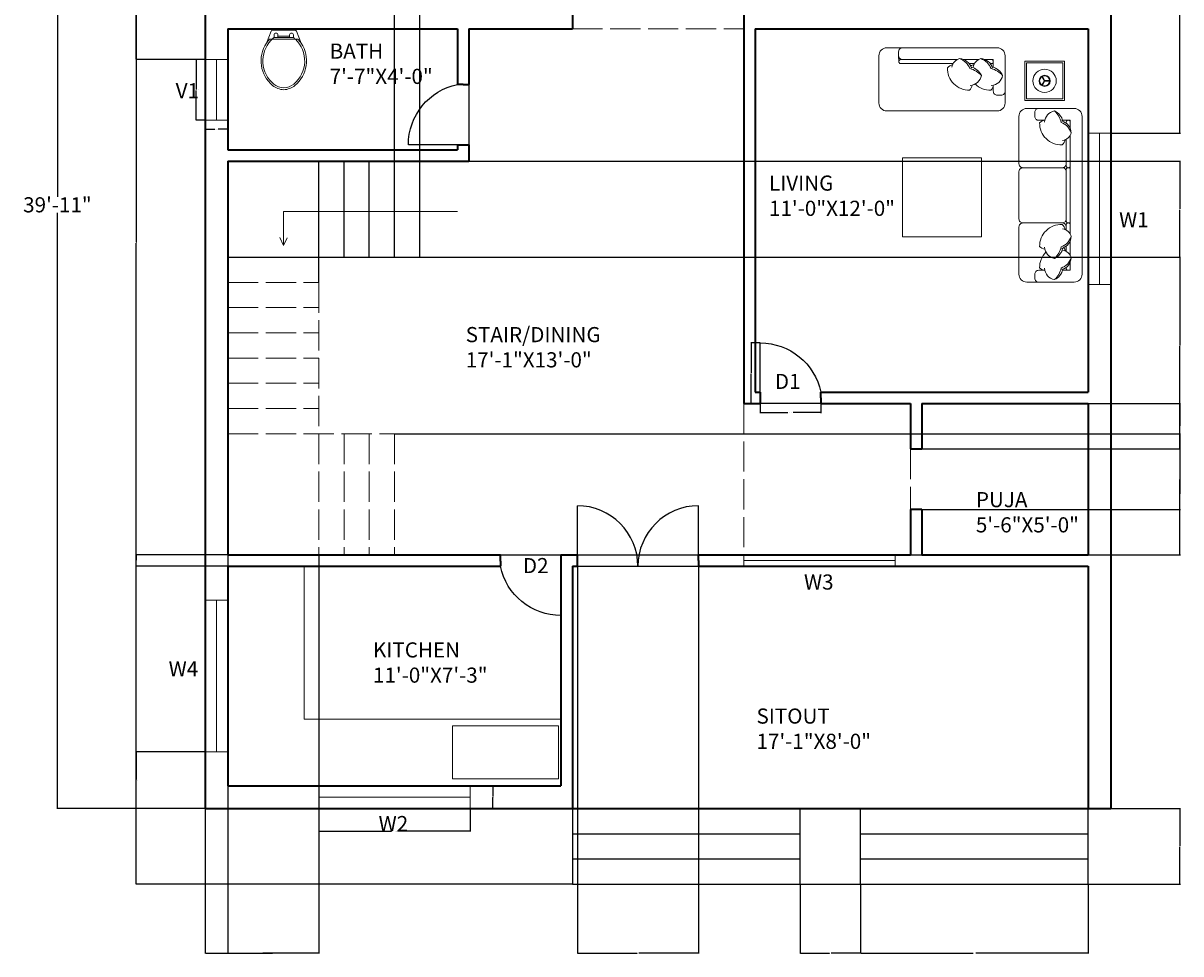
# Model space of a CAD drawing. Units: inches. Extents: x -53 to 406, y -526 to 46.
# Tile 1 of 2: x -53 to 406, y -526 to -157. Entities that reach past the tile are written whole.
import ezdxf

# ---------------------------------------------------------------- set-up
doc = ezdxf.new("R2010")
doc.units = ezdxf.units.IN
doc.header["$MEASUREMENT"] = 0
doc.linetypes.add('ACAD_ISO02W100', pattern=[15, 12, -3])
for name, color, linetype, lineweight in [('A-ANNO-DIMS', 2, 'Continuous', 18), ('A-ANNO-SYMB', 2, 'Continuous', 18), ('A-ANNO-TEXT', 7, 'Continuous', 18), ('A-AREA-IDEN', 7, 'Continuous', 25), ('A-DOOR', 40, 'Continuous', 25), ('A-FLOR-CASE', 9, 'Continuous', 18), ('A-FLOR-FIXT', 9, 'Continuous', 18), ('A-FLOR-STRS', 7, 'Continuous', 25), ('A-FLOR-STRS-OVHD', 7, 'ACAD_ISO02W100', 18), ('A-FURN', 8, 'Continuous', 13), ('A-GLAZ', 175, 'Continuous', 18), ('A-WALL', 7, 'Continuous', 35), ('A-WALL-OVHD', 7, 'ACAD_ISO02W100', 18), ('WC-Detail_dwgmodels.com', 251, 'Continuous', 13), ('WC-Outline_dwgmodels.com', 250, 'Continuous', 18)]:
    doc.layers.add(name, color=color, linetype=linetype, lineweight=lineweight)
doc.styles.get("Standard").update_dxf_attribs({"font": 'arial.ttf'})
doc.dimstyles.get("Standard").update_dxf_attribs({"dimtxt": 0.18, "dimasz": 0.18, "dimexe": 0.18, "dimexo": 0.0625, "dimgap": 0.09, "dimtad": 0, "dimtih": 1, "dimtoh": 1, "dimdec": 0, "dimzin": 0, "dimdsep": 46, "dimlunit": 3, "dimtxsty": 'Standard', "dimcen": 0.09, "dimadec": 0, "dimazin": 0, "dimtfac": 1, "dimtdec": 0, "dimtofl": 0, "dimtmove": 0, "dimatfit": 3, "dimfxl": 1, "dimtolj": 1, "dimtzin": 0, "dimarcsym": 0})

# ---------------------------------------------------------------- blocks, each defined once
blk = doc.blocks.new('*D2')
at = {"layer": 'A-ANNO-DIMS', "color": 0, "lineweight": -2, "transparency": 16777216}
for p, q in [((19.37, 9.91), (-39.35, 9.91)), ((-39.17, 9.73), (-39.17, -226.19)), ((-39.17, -468.41), (-39.17, -232.5)), ((19.37, -468.59), (-39.35, -468.59))]:
    blk.add_line(p, q, dxfattribs=at)
at = {"layer": 'A-ANNO-DIMS', "color": 0, "transparency": 16777216}
for points in [[(-39.2, 9.73), (-39.14, 9.73), (-39.17, 9.91)], [(-39.2, -468.41), (-39.14, -468.41), (-39.17, -468.59)]]:
    blk.add_solid(points, dxfattribs=at)
at = {"layer": 'Defpoints', "color": 0, "transparency": 16777216}
for p in [(19.43, 9.91), (-39.17, -468.59), (19.43, -468.59)]:
    blk.add_point(p, dxfattribs=at)
at = {"layer": 'A-ANNO-DIMS', "color": 0, "transparency": 16777216, "insert": (-39.17, -229.34), "char_height": 6, "attachment_point": 5}
blk.add_mtext('\\A1;39\'-11"', dxfattribs=at)
blk = doc.blocks.new('WIN-60IN-9IN-WALL')
for p, q in [((60, 9), (0, 9)), ((0, 9), (0, 0)), ((60, 0), (60, 9)), ((0, 4.5), (60, 4.5)), ((0, 0), (60, 0))]:
    blk.add_line(p, q)
blk = doc.blocks.new('VENT-24IN-9IN-WALL')
for p, q in [((24, 9), (0, 9)), ((0, 9), (0, 0)), ((24, 0), (24, 9)), ((0, 4.5), (24, 4.5)), ((0, 0), (24, 0))]:
    blk.add_line(p, q)
blk = doc.blocks.new('DOOR-24IN-SINGLE')
for p, q in [((24, 0), (24, 24)), ((0, 0), (24, 0))]:
    blk.add_line(p, q)
blk.add_arc((24, -0.52), 24.52, 90, 168.1877)
blk = doc.blocks.new('*D9')
at = {"layer": 'A-ANNO-DIMS', "color": 0, "lineweight": -2, "transparency": 16777216}
for p, q in [((64.43, -468.65), (64.43, -477.77)), ((124.43, -468.65), (124.43, -477.77)), ((64.61, -477.59), (93.2, -477.59)), ((124.25, -477.59), (95.66, -477.59))]:
    blk.add_line(p, q, dxfattribs=at)
at = {"layer": 'A-ANNO-DIMS', "color": 0, "transparency": 16777216}
for points in [[(64.61, -477.56), (64.61, -477.62), (64.43, -477.59)], [(124.25, -477.56), (124.25, -477.62), (124.43, -477.59)]]:
    blk.add_solid(points, dxfattribs=at)
at = {"layer": 'Defpoints', "color": 0, "transparency": 16777216}
for p in [(64.43, -468.59), (124.43, -468.59), (124.43, -477.59)]:
    blk.add_point(p, dxfattribs=at)
at = {"layer": 'A-ANNO-DIMS', "color": 0, "transparency": 16777216, "insert": (94.43, -477.59), "char_height": 0.18, "attachment_point": 5}
blk.add_mtext('\\A1;WINDOW 5\'-0" TYP.', dxfattribs=at)
blk = doc.blocks.new('*D10')
at = {"layer": 'A-ANNO-DIMS', "color": 0, "lineweight": -2, "transparency": 16777216}
for p, q in [((124.49, -459.59), (133.61, -459.59)), ((133.43, -459.77), (133.43, -463.91)), ((133.43, -468.41), (133.43, -464.27)), ((124.49, -468.59), (133.61, -468.59))]:
    blk.add_line(p, q, dxfattribs=at)
at = {"layer": 'A-ANNO-DIMS', "color": 0, "transparency": 16777216}
for points in [[(133.4, -459.77), (133.46, -459.77), (133.43, -459.59)], [(133.4, -468.41), (133.46, -468.41), (133.43, -468.59)]]:
    blk.add_solid(points, dxfattribs=at)
at = {"layer": 'Defpoints', "color": 0, "transparency": 16777216}
for p in [(124.43, -459.59), (133.43, -459.59), (124.43, -468.59)]:
    blk.add_point(p, dxfattribs=at)
at = {"layer": 'A-ANNO-DIMS', "color": 0, "transparency": 16777216, "insert": (133.43, -464.09), "char_height": 0.18, "attachment_point": 5}
blk.add_mtext('\\A1;0\'-9" TYP.', dxfattribs=at)
blk = doc.blocks.new('*D11')
at = {"layer": 'A-ANNO-DIMS', "color": 0, "lineweight": -2, "transparency": 16777216}
for p, q in [((239.43, -308.15), (239.43, -311.87)), ((239.61, -311.69), (250.38, -311.69)), ((263.25, -311.69), (252.48, -311.69)), ((263.43, -308.15), (263.43, -311.87))]:
    blk.add_line(p, q, dxfattribs=at)
at = {"layer": 'A-ANNO-DIMS', "color": 0, "transparency": 16777216}
for points in [[(239.61, -311.66), (239.61, -311.72), (239.43, -311.69)], [(263.25, -311.66), (263.25, -311.72), (263.43, -311.69)]]:
    blk.add_solid(points, dxfattribs=at)
at = {"layer": 'Defpoints', "color": 0, "transparency": 16777216}
for p in [(239.43, -308.09), (239.43, -311.69), (263.43, -308.09)]:
    blk.add_point(p, dxfattribs=at)
at = {"layer": 'A-ANNO-DIMS', "color": 0, "transparency": 16777216, "insert": (251.43, -311.69), "char_height": 0.18, "attachment_point": 5}
blk.add_mtext('\\A1;DOOR 2\'-0" TYP.', dxfattribs=at)
blk = doc.blocks.new('*D12')
at = {"layer": 'A-ANNO-DIMS', "color": 0, "lineweight": -2, "transparency": 16777216}
for p, q in [((239.37, -284.09), (235.65, -284.09)), ((235.83, -284.27), (235.83, -295.91)), ((235.83, -307.91), (235.83, -296.27)), ((239.37, -308.09), (235.65, -308.09))]:
    blk.add_line(p, q, dxfattribs=at)
at = {"layer": 'A-ANNO-DIMS', "color": 0, "transparency": 16777216}
for points in [[(235.8, -284.27), (235.86, -284.27), (235.83, -284.09)], [(235.8, -307.91), (235.86, -307.91), (235.83, -308.09)]]:
    blk.add_solid(points, dxfattribs=at)
at = {"layer": 'Defpoints', "color": 0, "transparency": 16777216}
for p in [(235.83, -284.09), (239.43, -284.09), (239.43, -308.09)]:
    blk.add_point(p, dxfattribs=at)
at = {"layer": 'A-ANNO-DIMS', "color": 0, "transparency": 16777216, "insert": (235.83, -296.09), "char_height": 0.18, "attachment_point": 5}
blk.add_mtext('\\A1;2\'-0" TYP.', dxfattribs=at)
blk = doc.blocks.new('*D13')
at = {"layer": 'A-ANNO-DIMS', "color": 0, "lineweight": -2, "transparency": 16777216}
for p, q in [((19.37, -171.79), (15.65, -171.79)), ((15.83, -171.97), (15.83, -183.61)), ((15.83, -195.61), (15.83, -183.97)), ((19.37, -195.79), (15.65, -195.79))]:
    blk.add_line(p, q, dxfattribs=at)
at = {"layer": 'A-ANNO-DIMS', "color": 0, "transparency": 16777216}
for points in [[(15.8, -171.97), (15.86, -171.97), (15.83, -171.79)], [(15.8, -195.61), (15.86, -195.61), (15.83, -195.79)]]:
    blk.add_solid(points, dxfattribs=at)
at = {"layer": 'Defpoints', "color": 0, "transparency": 16777216}
for p in [(15.83, -171.79), (19.43, -171.79), (19.43, -195.79)]:
    blk.add_point(p, dxfattribs=at)
at = {"layer": 'A-ANNO-DIMS', "color": 0, "transparency": 16777216, "insert": (15.83, -183.79), "char_height": 0.18, "attachment_point": 5}
blk.add_mtext('\\A1;VENT 2\'-0" TYP.', dxfattribs=at)
blk = doc.blocks.new('*D14')
at = {"layer": 'A-ANNO-DIMS', "color": 0, "lineweight": -2, "transparency": 16777216}
for p, q in [((19.43, -195.86), (19.43, -199.57)), ((28.43, -195.86), (28.43, -199.57)), ((19.61, -199.39), (23.29, -199.39)), ((28.25, -199.39), (24.57, -199.39))]:
    blk.add_line(p, q, dxfattribs=at)
at = {"layer": 'A-ANNO-DIMS', "color": 0, "transparency": 16777216}
for points in [[(19.61, -199.36), (19.61, -199.42), (19.43, -199.39)], [(28.25, -199.36), (28.25, -199.42), (28.43, -199.39)]]:
    blk.add_solid(points, dxfattribs=at)
at = {"layer": 'Defpoints', "color": 0, "transparency": 16777216}
for p in [(19.43, -195.79), (28.43, -195.79), (19.43, -199.39)]:
    blk.add_point(p, dxfattribs=at)
at = {"layer": 'A-ANNO-DIMS', "color": 0, "transparency": 16777216, "insert": (23.93, -199.39), "char_height": 0.18, "attachment_point": 5}
blk.add_mtext('\\A1;0\'-9" TYP.', dxfattribs=at)
blk = doc.blocks.new('*D21')
at = {"layer": 'A-ANNO-DIMS', "color": 0, "lineweight": -2, "transparency": 16777216}
for p, q in [((378.49, -468.59), (405.96, -468.59)), ((405.78, -468.77), (405.78, -483.41)), ((405.78, -498.41), (405.78, -483.77)), ((369.49, -498.59), (405.96, -498.59))]:
    blk.add_line(p, q, dxfattribs=at)
at = {"layer": 'A-ANNO-DIMS', "color": 0, "transparency": 16777216}
for points in [[(405.75, -468.77), (405.81, -468.77), (405.78, -468.59)], [(405.75, -498.41), (405.81, -498.41), (405.78, -498.59)]]:
    blk.add_solid(points, dxfattribs=at)
at = {"layer": 'Defpoints', "color": 0, "transparency": 16777216}
for p in [(378.43, -468.59), (369.43, -498.59), (405.78, -498.59)]:
    blk.add_point(p, dxfattribs=at)
at = {"layer": 'A-ANNO-DIMS', "color": 0, "transparency": 16777216, "insert": (405.78, -483.59), "char_height": 0.18, "attachment_point": 5}
blk.add_mtext('\\A1;2\'-6"', dxfattribs=at)
blk = doc.blocks.new('*D26')
at = {"layer": 'A-ANNO-DIMS', "color": 0, "lineweight": -2, "transparency": 16777216}
for p, q in [((378.49, -107.09), (405.96, -107.09)), ((405.78, -107.27), (405.78, -153.82)), ((405.78, -200.73), (405.78, -154.18)), ((378.49, -200.91), (405.96, -200.91))]:
    blk.add_line(p, q, dxfattribs=at)
at = {"layer": 'A-ANNO-DIMS', "color": 0, "transparency": 16777216}
for points in [[(405.75, -107.27), (405.81, -107.27), (405.78, -107.09)], [(405.75, -200.73), (405.81, -200.73), (405.78, -200.91)]]:
    blk.add_solid(points, dxfattribs=at)
at = {"layer": 'Defpoints', "color": 0, "transparency": 16777216}
for p in [(378.43, -107.09), (378.43, -200.91), (405.78, -200.91)]:
    blk.add_point(p, dxfattribs=at)
at = {"layer": 'A-ANNO-DIMS', "color": 0, "transparency": 16777216, "insert": (405.78, -154), "char_height": 0.18, "attachment_point": 5}
blk.add_mtext('\\A1;7\'-10"', dxfattribs=at)
blk = doc.blocks.new('*D27')
at = {"layer": 'A-ANNO-DIMS', "color": 0, "lineweight": -2, "transparency": 16777216}
for p, q in [((19.37, -107.09), (-8.1, -107.09)), ((-7.92, -107.27), (-7.92, -139.26)), ((-7.92, -171.61), (-7.92, -139.63)), ((19.37, -171.79), (-8.1, -171.79))]:
    blk.add_line(p, q, dxfattribs=at)
at = {"layer": 'A-ANNO-DIMS', "color": 0, "transparency": 16777216}
for points in [[(-7.95, -107.27), (-7.89, -107.27), (-7.92, -107.09)], [(-7.95, -171.61), (-7.89, -171.61), (-7.92, -171.79)]]:
    blk.add_solid(points, dxfattribs=at)
at = {"layer": 'Defpoints', "color": 0, "transparency": 16777216}
for p in [(19.43, -107.09), (-7.92, -171.79), (19.43, -171.79)]:
    blk.add_point(p, dxfattribs=at)
at = {"layer": 'A-ANNO-DIMS', "color": 0, "transparency": 16777216, "insert": (-7.92, -139.44), "char_height": 0.18, "attachment_point": 5}
blk.add_mtext('\\A1;5\'-4 1/2"', dxfattribs=at)
blk = doc.blocks.new('*D28')
at = {"layer": 'A-ANNO-DIMS', "color": 0, "lineweight": -2, "transparency": 16777216}
for p, q in [((19.37, -446.09), (-8.1, -446.09)), ((-7.92, -446.27), (-7.92, -457.16)), ((-7.92, -468.41), (-7.92, -457.52)), ((19.37, -468.59), (-8.1, -468.59))]:
    blk.add_line(p, q, dxfattribs=at)
at = {"layer": 'A-ANNO-DIMS', "color": 0, "transparency": 16777216}
for points in [[(-7.95, -446.27), (-7.89, -446.27), (-7.92, -446.09)], [(-7.95, -468.41), (-7.89, -468.41), (-7.92, -468.59)]]:
    blk.add_solid(points, dxfattribs=at)
at = {"layer": 'Defpoints', "color": 0, "transparency": 16777216}
for p in [(-7.92, -446.09), (19.43, -446.09), (19.43, -468.59)]:
    blk.add_point(p, dxfattribs=at)
at = {"layer": 'A-ANNO-DIMS', "color": 0, "transparency": 16777216, "insert": (-7.92, -457.34), "char_height": 0.18, "attachment_point": 5}
blk.add_mtext('\\A1;1\'-10 1/2"', dxfattribs=at)
blk = doc.blocks.new('*D29')
at = {"layer": 'A-ANNO-DIMS', "color": 0, "lineweight": -2, "transparency": 16777216}
for p, q in [((166.93, -372.65), (166.93, -526.12)), ((214.93, -372.65), (214.93, -526.12)), ((167.11, -525.94), (190.6, -525.94)), ((214.75, -525.94), (191.26, -525.94))]:
    blk.add_line(p, q, dxfattribs=at)
at = {"layer": 'A-ANNO-DIMS', "color": 0, "transparency": 16777216}
for points in [[(167.11, -525.91), (167.11, -525.97), (166.93, -525.94)], [(214.75, -525.91), (214.75, -525.97), (214.93, -525.94)]]:
    blk.add_solid(points, dxfattribs=at)
at = {"layer": 'Defpoints', "color": 0, "transparency": 16777216}
for p in [(166.93, -372.59), (214.93, -372.59), (214.93, -525.94)]:
    blk.add_point(p, dxfattribs=at)
at = {"layer": 'A-ANNO-DIMS', "color": 0, "transparency": 16777216, "insert": (190.93, -525.94), "char_height": 0.18, "attachment_point": 5}
blk.add_mtext('\\A1;4\'-0"', dxfattribs=at)
blk = doc.blocks.new('*D30')
at = {"layer": 'A-ANNO-DIMS', "color": 0, "lineweight": -2, "transparency": 16777216}
for p, q in [((19.43, -468.65), (19.43, -526.12)), ((64.43, -468.65), (64.43, -526.12)), ((19.61, -525.94), (41.6, -525.94)), ((64.25, -525.94), (42.26, -525.94))]:
    blk.add_line(p, q, dxfattribs=at)
at = {"layer": 'A-ANNO-DIMS', "color": 0, "transparency": 16777216}
for points in [[(19.61, -525.91), (19.61, -525.97), (19.43, -525.94)], [(64.25, -525.91), (64.25, -525.97), (64.43, -525.94)]]:
    blk.add_solid(points, dxfattribs=at)
at = {"layer": 'Defpoints', "color": 0, "transparency": 16777216}
for p in [(19.43, -468.59), (64.43, -468.59), (64.43, -525.94)]:
    blk.add_point(p, dxfattribs=at)
at = {"layer": 'A-ANNO-DIMS', "color": 0, "transparency": 16777216, "insert": (41.93, -525.94), "char_height": 0.18, "attachment_point": 5}
blk.add_mtext('\\A1;3\'-9"', dxfattribs=at)
blk = doc.blocks.new('*D31')
at = {"layer": 'A-ANNO-DIMS', "color": 0, "lineweight": -2, "transparency": 16777216}
for p, q in [((255.18, -498.65), (255.18, -526.12)), ((279.18, -498.65), (279.18, -526.12)), ((255.36, -525.94), (266.85, -525.94)), ((279, -525.94), (267.51, -525.94))]:
    blk.add_line(p, q, dxfattribs=at)
at = {"layer": 'A-ANNO-DIMS', "color": 0, "transparency": 16777216}
for points in [[(255.36, -525.91), (255.36, -525.97), (255.18, -525.94)], [(279, -525.91), (279, -525.97), (279.18, -525.94)]]:
    blk.add_solid(points, dxfattribs=at)
at = {"layer": 'Defpoints', "color": 0, "transparency": 16777216}
for p in [(255.18, -498.59), (279.18, -498.59), (279.18, -525.94)]:
    blk.add_point(p, dxfattribs=at)
at = {"layer": 'A-ANNO-DIMS', "color": 0, "transparency": 16777216, "insert": (267.18, -525.94), "char_height": 0.18, "attachment_point": 5}
blk.add_mtext('\\A1;2\'-0"', dxfattribs=at)
blk = doc.blocks.new('*D32')
at = {"layer": 'A-ANNO-DIMS', "color": 0, "lineweight": -2, "transparency": 16777216}
for p, q in [((279.18, -498.65), (279.18, -526.12)), ((369.43, -498.65), (369.43, -526.12)), ((279.36, -525.94), (323.77, -525.94)), ((369.25, -525.94), (324.84, -525.94))]:
    blk.add_line(p, q, dxfattribs=at)
at = {"layer": 'A-ANNO-DIMS', "color": 0, "transparency": 16777216}
for points in [[(279.36, -525.91), (279.36, -525.97), (279.18, -525.94)], [(369.25, -525.91), (369.25, -525.97), (369.43, -525.94)]]:
    blk.add_solid(points, dxfattribs=at)
at = {"layer": 'Defpoints', "color": 0, "transparency": 16777216}
for p in [(279.18, -498.59), (369.43, -498.59), (369.43, -525.94)]:
    blk.add_point(p, dxfattribs=at)
at = {"layer": 'A-ANNO-DIMS', "color": 0, "transparency": 16777216, "insert": (324.31, -525.94), "char_height": 0.18, "attachment_point": 5}
blk.add_mtext('\\A1;7\'-6 1/2"', dxfattribs=at)
blk = doc.blocks.new('*D33')
at = {"layer": 'A-ANNO-DIMS', "color": 0, "lineweight": -2, "transparency": 16777216}
for p, q in [((19.37, 9.91), (-8.1, 9.91)), ((-7.92, 9.73), (-7.92, -244.16)), ((-7.92, -498.41), (-7.92, -244.52)), ((164.87, -498.59), (-8.1, -498.59))]:
    blk.add_line(p, q, dxfattribs=at)
at = {"layer": 'A-ANNO-DIMS', "color": 0, "transparency": 16777216}
for points in [[(-7.95, 9.73), (-7.89, 9.73), (-7.92, 9.91)], [(-7.95, -498.41), (-7.89, -498.41), (-7.92, -498.59)]]:
    blk.add_solid(points, dxfattribs=at)
at = {"layer": 'Defpoints', "color": 0, "transparency": 16777216}
for p in [(19.43, 9.91), (-7.92, -498.59), (164.93, -498.59)]:
    blk.add_point(p, dxfattribs=at)
at = {"layer": 'A-ANNO-DIMS', "color": 0, "transparency": 16777216, "insert": (-7.92, -244.34), "char_height": 0.18, "attachment_point": 5}
blk.add_mtext('\\A1;42\'-4 1/2"', dxfattribs=at)
blk = doc.blocks.new('*D34')
at = {"layer": 'A-ANNO-DIMS', "color": 0, "lineweight": -2, "transparency": 16777216}
for p, q in [((104.49, -212.09), (405.96, -212.09)), ((405.78, -212.27), (405.78, -230.91)), ((405.78, -249.91), (405.78, -231.27)), ((104.49, -250.09), (405.96, -250.09))]:
    blk.add_line(p, q, dxfattribs=at)
at = {"layer": 'A-ANNO-DIMS', "color": 0, "transparency": 16777216}
for points in [[(405.75, -212.27), (405.81, -212.27), (405.78, -212.09)], [(405.75, -249.91), (405.81, -249.91), (405.78, -250.09)]]:
    blk.add_solid(points, dxfattribs=at)
at = {"layer": 'Defpoints', "color": 0, "transparency": 16777216}
for p in [(104.43, -212.09), (104.43, -250.09), (405.78, -250.09)]:
    blk.add_point(p, dxfattribs=at)
at = {"layer": 'A-ANNO-DIMS', "color": 0, "transparency": 16777216, "insert": (405.78, -231.09), "char_height": 0.18, "attachment_point": 5}
blk.add_mtext('\\A1;3\'-2"', dxfattribs=at)
blk = doc.blocks.new('*D35')
at = {"layer": 'A-ANNO-DIMS', "color": 0, "lineweight": -2, "transparency": 16777216}
for p, q in [((28.43, -368.15), (28.43, -526.12)), ((64.43, -368.15), (64.43, -526.12)), ((28.61, -525.94), (46.1, -525.94)), ((64.25, -525.94), (46.76, -525.94))]:
    blk.add_line(p, q, dxfattribs=at)
at = {"layer": 'A-ANNO-DIMS', "color": 0, "transparency": 16777216}
for points in [[(28.61, -525.91), (28.61, -525.97), (28.43, -525.94)], [(64.25, -525.91), (64.25, -525.97), (64.43, -525.94)]]:
    blk.add_solid(points, dxfattribs=at)
at = {"layer": 'Defpoints', "color": 0, "transparency": 16777216}
for p in [(28.43, -368.09), (64.43, -368.09), (64.43, -525.94)]:
    blk.add_point(p, dxfattribs=at)
at = {"layer": 'A-ANNO-DIMS', "color": 0, "transparency": 16777216, "insert": (46.43, -525.94), "char_height": 0.18, "attachment_point": 5}
blk.add_mtext('\\A1;3\'-0"', dxfattribs=at)
blk = doc.blocks.new('*D36')
at = {"layer": 'A-ANNO-DIMS', "color": 0, "lineweight": -2, "transparency": 16777216}
for p, q in [((94.49, -320.09), (405.96, -320.09)), ((405.78, -320.27), (405.78, -343.91)), ((405.78, -367.91), (405.78, -344.27)), ((94.49, -368.09), (405.96, -368.09))]:
    blk.add_line(p, q, dxfattribs=at)
at = {"layer": 'A-ANNO-DIMS', "color": 0, "transparency": 16777216}
for points in [[(405.75, -320.27), (405.81, -320.27), (405.78, -320.09)], [(405.75, -367.91), (405.81, -367.91), (405.78, -368.09)]]:
    blk.add_solid(points, dxfattribs=at)
at = {"layer": 'Defpoints', "color": 0, "transparency": 16777216}
for p in [(94.43, -320.09), (405.78, -320.09), (94.43, -368.09)]:
    blk.add_point(p, dxfattribs=at)
at = {"layer": 'A-ANNO-DIMS', "color": 0, "transparency": 16777216, "insert": (405.78, -344.09), "char_height": 0.18, "attachment_point": 5}
blk.add_mtext('\\A1;4\'-0"', dxfattribs=at)
blk = doc.blocks.new('*D37')
at = {"layer": 'A-ANNO-DIMS', "color": 0, "lineweight": -2, "transparency": 16777216}
for p, q in [((104.49, -250.09), (405.96, -250.09)), ((405.78, -250.27), (405.78, -284.91)), ((405.78, -319.91), (405.78, -285.27)), ((94.49, -320.09), (405.96, -320.09))]:
    blk.add_line(p, q, dxfattribs=at)
at = {"layer": 'A-ANNO-DIMS', "color": 0, "transparency": 16777216}
for points in [[(405.75, -250.27), (405.81, -250.27), (405.78, -250.09)], [(405.75, -319.91), (405.81, -319.91), (405.78, -320.09)]]:
    blk.add_solid(points, dxfattribs=at)
at = {"layer": 'Defpoints', "color": 0, "transparency": 16777216}
for p in [(104.43, -250.09), (94.43, -320.09), (405.78, -320.09)]:
    blk.add_point(p, dxfattribs=at)
at = {"layer": 'A-ANNO-DIMS', "color": 0, "transparency": 16777216, "insert": (405.78, -285.09), "char_height": 0.18, "attachment_point": 5}
blk.add_mtext('\\A1;5\'-10"', dxfattribs=at)
blk = doc.blocks.new('*D38')
at = {"layer": 'A-ANNO-DIMS', "color": 0, "lineweight": -2, "transparency": 16777216}
for p, q in [((94.43, -212.03), (94.43, 37.44)), ((94.61, 37.26), (99.03, 37.26)), ((104.25, 37.26), (99.83, 37.26)), ((104.43, -212.03), (104.43, 37.44))]:
    blk.add_line(p, q, dxfattribs=at)
at = {"layer": 'A-ANNO-DIMS', "color": 0, "transparency": 16777216}
for points in [[(94.61, 37.29), (94.61, 37.23), (94.43, 37.26)], [(104.25, 37.29), (104.25, 37.23), (104.43, 37.26)]]:
    blk.add_solid(points, dxfattribs=at)
at = {"layer": 'Defpoints', "color": 0, "transparency": 16777216}
for p in [(104.43, 37.26), (94.43, -212.09), (104.43, -212.09)]:
    blk.add_point(p, dxfattribs=at)
at = {"layer": 'A-ANNO-DIMS', "color": 0, "transparency": 16777216, "insert": (99.43, 37.26), "char_height": 0.18, "attachment_point": 5}
blk.add_mtext('\\A1;0\'-10"', dxfattribs=at)
blk = doc.blocks.new('*D39')
at = {"layer": 'A-ANNO-DIMS', "color": 0, "lineweight": -2, "transparency": 16777216}
for p, q in [((28.37, -368.09), (-8.1, -368.09)), ((-7.92, -368.27), (-7.92, -370.16)), ((-7.92, -372.41), (-7.92, -370.52)), ((28.37, -372.59), (-8.1, -372.59))]:
    blk.add_line(p, q, dxfattribs=at)
at = {"layer": 'A-ANNO-DIMS', "color": 0, "transparency": 16777216}
for points in [[(-7.95, -368.27), (-7.89, -368.27), (-7.92, -368.09)], [(-7.95, -372.41), (-7.89, -372.41), (-7.92, -372.59)]]:
    blk.add_solid(points, dxfattribs=at)
at = {"layer": 'Defpoints', "color": 0, "transparency": 16777216}
for p in [(28.43, -368.09), (-7.92, -372.59), (28.43, -372.59)]:
    blk.add_point(p, dxfattribs=at)
at = {"layer": 'A-ANNO-DIMS', "color": 0, "transparency": 16777216, "insert": (-7.92, -370.34), "char_height": 0.18, "attachment_point": 5}
blk.add_mtext('\\A1;0\'-4 1/2"', dxfattribs=at)
blk = doc.blocks.new('*D40')
at = {"layer": 'A-ANNO-DIMS', "color": 0, "lineweight": -2, "transparency": 16777216}
for p, q in [((303.49, -326.09), (405.96, -326.09)), ((405.78, -326.27), (405.78, -337.91)), ((405.78, -349.91), (405.78, -338.27)), ((303.49, -350.09), (405.96, -350.09))]:
    blk.add_line(p, q, dxfattribs=at)
at = {"layer": 'A-ANNO-DIMS', "color": 0, "transparency": 16777216}
for points in [[(405.75, -326.27), (405.81, -326.27), (405.78, -326.09)], [(405.75, -349.91), (405.81, -349.91), (405.78, -350.09)]]:
    blk.add_solid(points, dxfattribs=at)
at = {"layer": 'Defpoints', "color": 0, "transparency": 16777216}
for p in [(303.43, -326.09), (303.43, -350.09), (405.78, -350.09)]:
    blk.add_point(p, dxfattribs=at)
at = {"layer": 'A-ANNO-DIMS', "color": 0, "transparency": 16777216, "insert": (405.78, -338.09), "char_height": 0.18, "attachment_point": 5}
blk.add_mtext('\\A1;2\'-0"', dxfattribs=at)
blk = doc.blocks.new('*D41')
at = {"layer": 'A-ANNO-DIMS', "color": 0, "lineweight": -2, "transparency": 16777216}
for p, q in [((303.49, -308.09), (405.96, -308.09)), ((405.78, -308.27), (405.78, -316.91)), ((405.78, -325.91), (405.78, -317.27)), ((303.49, -326.09), (405.96, -326.09))]:
    blk.add_line(p, q, dxfattribs=at)
at = {"layer": 'A-ANNO-DIMS', "color": 0, "transparency": 16777216}
for points in [[(405.75, -308.27), (405.81, -308.27), (405.78, -308.09)], [(405.75, -325.91), (405.81, -325.91), (405.78, -326.09)]]:
    blk.add_solid(points, dxfattribs=at)
at = {"layer": 'Defpoints', "color": 0, "transparency": 16777216}
for p in [(303.43, -308.09), (303.43, -326.09), (405.78, -326.09)]:
    blk.add_point(p, dxfattribs=at)
at = {"layer": 'A-ANNO-DIMS', "color": 0, "transparency": 16777216, "insert": (405.78, -317.09), "char_height": 0.18, "attachment_point": 5}
blk.add_mtext('\\A1;1\'-6"', dxfattribs=at)

msp = doc.modelspace()

# ---------------------------------------------------------------- linework, layer by layer
at = {"layer": 'A-ANNO-SYMB'}
for p, q in [((119.47, -232.03), (50.5, -232.03)), ((50.5, -232.03), (50.5, -245.41)), ((50.5, -245.41), (48.99, -242.29)), ((50.5, -245.41), (51.89, -242.43))]:
    msp.add_line(p, q, dxfattribs=at)
at = {"layer": 'A-DOOR'}
for p, q in [((166.93, -372.59), (166.93, -348.59)), ((214.93, -372.59), (214.93, -348.59)), ((166.93, -372.59), (214.93, -372.59))]:
    msp.add_line(p, q, dxfattribs=at)
for centre, start, end in [((166.93, -372.59), 0, 90), ((214.93, -372.59), 90, 180)]:
    msp.add_arc(centre, 24, start, end, dxfattribs=at)
at = {"layer": 'A-FLOR-CASE'}
for p, q in [((58.7, -372.59), (58.7, -433.25)), ((58.7, -433.25), (160.43, -433.25))]:
    msp.add_line(p, q, dxfattribs=at)
at = {"layer": 'A-FLOR-FIXT'}
for p, q in [((117.39, -435.78), (117.39, -456.8)), ((159.43, -435.78), (117.39, -435.78)), ((159.43, -456.8), (159.43, -435.78)), ((117.39, -456.8), (159.43, -456.8))]:
    msp.add_line(p, q, dxfattribs=at)
at = {"layer": 'A-FLOR-STRS'}
for p, q in [((64.43, -260.09), (64.43, -212.09)), ((74.43, -250.09), (74.43, -212.09)), ((84.43, -250.09), (84.43, -212.09)), ((94.43, -250.09), (94.43, -212.09)), ((104.43, -250.09), (104.43, -212.09)), ((28.43, -250.09), (104.43, -250.09)), ((164.93, -468.59), (164.93, -478.59)), ((255.18, -498.59), (255.18, -468.59)), ((279.18, -498.59), (279.18, -468.59)), ((369.43, -498.59), (369.43, -468.59)), ((164.93, -478.59), (164.93, -488.59)), ((164.93, -478.59), (255.18, -478.59)), ((279.18, -478.59), (369.43, -478.59)), ((164.93, -488.59), (164.93, -498.59)), ((164.93, -488.59), (255.18, -488.59)), ((279.18, -488.59), (369.43, -488.59)), ((164.93, -498.59), (369.43, -498.59))]:
    msp.add_line(p, q, dxfattribs=at)
at = {"layer": 'A-FLOR-STRS-OVHD'}
for p, q in [((28.43, -260.09), (64.43, -260.09)), ((64.43, -260.09), (64.43, -368.09)), ((28.43, -270.09), (64.43, -270.09)), ((28.43, -280.09), (64.43, -280.09)), ((28.43, -290.09), (64.43, -290.09)), ((28.43, -300.09), (64.43, -300.09)), ((28.43, -310.09), (64.43, -310.09)), ((28.43, -320.09), (94.43, -320.09)), ((74.43, -320.09), (74.43, -368.09)), ((84.43, -320.09), (84.43, -368.09)), ((94.43, -320.09), (94.43, -368.09))]:
    msp.add_line(p, q, dxfattribs=at)
at = {"layer": 'A-FURN'}
for p, q in [((294.25, -170.24), (294.4, -172.59)), ((352.04, -180.26), (350.93, -178.34)), ((352.21, -180.16), (351.11, -178.25)), ((352.04, -180.16), (350.93, -182.07)), ((352.21, -180.26), (351.11, -182.17)), ((352.12, -180.11), (354.33, -180.11)), ((352.12, -180.3), (354.33, -180.3))]:
    msp.add_line(p, q, dxfattribs=at)
at = {"layer": 'A-FURN', "ltscale": 0.03}
for points in [[(286.43, -189.01, 0.414214), (289.55, -192.14), (289.55, -192.14, -0.317837), (289.55, -192.14, 0.414214), (289.55, -192.14), (289.55, -192.14, -1.186185), (289.55, -192.14, 0.414214), (289.55, -192.14), (333.35, -192.14, 0.414214), (336.48, -189.01), (336.48, -170.24, 0.414214), (333.35, -167.11), (289.55, -167.11, 0.414214), (286.43, -170.24)], [(345.08, -191.16, 0.414214), (341.96, -194.28), (341.96, -213.05, 0.414214), (343.52, -214.62, 0.414214), (341.96, -216.18), (341.96, -234.95, 0.414214), (343.52, -236.52, 0.414214), (341.96, -238.08), (341.96, -256.85, 0.414214), (345.08, -259.98), (363.85, -259.98, 0.414214), (366.98, -256.85), (366.98, -194.28, 0.414214), (363.85, -191.16)]]:
    msp.add_lwpolyline(points, format="xyb", close=True, dxfattribs=at)
at = {"layer": 'A-FURN'}
for points in [[(298.23, -171.8), (295.81, -171.8, -0.414214), (294.25, -170.24), (294.25, -168.67, -0.414214), (295.81, -167.11)], [(317.47, -171.8), (295.02, -171.8, 0.414214), (294.4, -172.43), (294.4, -172.74, 0.414214), (295.02, -173.37), (315.89, -173.37, 0.414214)], [(323.37, -181.89, -0.165541), (322.4, -183.96, -0.425989), (313.61, -175, -0.121523), (315.7, -173.76, 7.115464)], [(323.12, -175.14, 0.306663), (318.45, -171.41, 0.30633), (315.41, -174.82, -0.872847)], [(327.06, -178.05, 0.14773), (322.49, -175.36, 0.213343), (318.45, -171.41, 0.178662)], [(325.9, -171.8), (320.07, -171.8, 0.414214)], [(322.17, -173.37), (324.32, -173.37, 0.414214)], [(322.81, -174.38, -0.071865), (324.12, -173.76, 7.115464)], [(331.55, -175.14, 0.306663), (326.88, -171.41, 0.30633), (323.83, -174.82, -0.872847)], [(335.49, -178.05, 0.14773), (330.91, -175.36, 0.213343), (326.88, -171.41, 0.178662)], [(331.16, -171.8), (328.5, -171.8, 0.414214)], [(328.5, -171.8), (331.79, -171.8), (331.79, -174.88, 0.414214)], [(330.59, -173.37), (331.16, -173.37, 0.414214), (331.79, -172.74), (331.79, -172.43, 0.414214), (331.16, -171.8)], [(322.58, -181.99, 0.356772), (327.06, -178.05, 0.249542), (323, -174.8, -9.61688)], [(331, -181.99, 0.356772), (335.49, -178.05, 0.249542), (331.42, -174.8, -9.61688)], [(331.79, -181.89, -0.165541), (330.82, -183.96, -0.200231), (324.61, -181.44, -0.121523)], [(331.79, -181.89), (331.79, -184.32, 0.414214), (333.35, -185.88), (334.92, -185.88, 0.414214), (336.48, -184.32)], [(349.78, -191.16, 0.414214), (348.21, -192.72), (348.21, -194.28, 0.414214), (349.78, -195.85), (352.2, -195.85)], [(352.11, -196.63, -0.356772), (356.05, -192.15, -0.249542), (359.3, -196.21)], [(356.05, -192.15, -0.14773), (358.74, -196.72, -0.213343), (362.68, -200.76)], [(352.2, -195.84, 0.165541), (350.13, -196.81, 0.425989), (359.09, -205.6, 0.121523), (360.33, -203.51)], [(358.95, -196.09, -0.306663), (362.68, -200.76, -0.30633), (359.27, -203.8)], [(360.73, -197.04), (360.73, -196.47, -0.414214), (361.35, -195.85), (361.66, -195.85, -0.414214), (362.29, -196.47)], [(362.29, -196.47), (362.29, -199.14, -0.412535)], [(362.29, -201.74), (362.29, -213.99, -0.414214), (361.66, -214.62), (361.35, -214.62, -0.414214), (360.73, -213.99), (360.73, -203.32, -0.412652)], [(360.73, -213.05, -0.414214), (359.16, -214.62), (343.52, -214.62, -0.415249)], [(360.73, -216.18, 0.414214), (359.16, -214.62)], [(360.73, -238.08, 0.414214), (359.16, -236.52), (343.52, -236.52, 0.41732)], [(352.2, -246.86, -0.165541), (350.13, -245.9, -0.425989), (359.09, -237.11, -0.121523), (360.33, -239.2)], [(360.73, -234.95, -0.414214), (359.16, -236.52)], [(362.29, -240.97), (362.29, -237.14, 0.414214), (361.66, -236.52), (361.35, -236.52, 0.414214), (360.73, -237.14), (360.73, -239.39, 0.126313)], [(356.05, -250.56, 0.14773), (358.74, -245.99, 0.213343), (362.68, -241.95)], [(358.95, -246.62, 0.306663), (362.68, -241.95, 0.30633), (359.27, -238.9)], [(352.11, -246.08, 0.356772), (356.05, -250.56, 0.249542), (359.3, -246.5)], [(358.95, -255.04, 0.306663), (362.68, -250.38, 0.30633), (359.27, -247.33)], [(359.72, -246.31, -0.071865), (360.33, -247.62)], [(360.73, -245.67), (360.73, -247.82, 0.414599)], [(362.29, -249.39), (362.29, -243.57, 0.414747)], [(352.2, -255.29, -0.165541), (350.13, -254.32, -0.200231), (352.65, -248.11)], [(356.05, -258.98, 0.14773), (358.74, -254.41, 0.213343), (362.68, -250.38)], [(362.29, -252), (362.29, -255.29), (359.22, -255.29, 0.414352)], [(362.29, -254.66), (362.29, -252, 0.414469)], [(352.2, -255.29), (349.78, -255.29, 0.414214), (348.21, -256.85), (348.21, -258.42, 0.414214), (349.78, -259.98)], [(352.11, -254.5, 0.356772), (356.05, -258.98, 0.249542), (359.3, -254.92)], [(360.73, -254.09), (360.73, -254.66, 0.414214), (361.35, -255.29), (361.66, -255.29, 0.414214), (362.29, -254.66)]]:
    msp.add_lwpolyline(points, format="xyb", dxfattribs=at)
for points in [[(298.23, -171.8), (317.47, -171.8)], [(320.07, -171.8), (325.9, -171.8)], [(359.22, -195.85), (362.29, -195.85), (362.29, -199.14)], [(362.29, -201.74), (362.29, -240.97)], [(362.29, -243.57), (362.29, -249.39)]]:
    msp.add_lwpolyline(points, dxfattribs=at)
at = {"layer": 'A-FURN', "ltscale": 0.03}
for points in [[(344.3, -172.38), (344.3, -188.03), (359.94, -188.03), (359.94, -172.38)], [(295.81, -241.99), (295.81, -210.71), (327.1, -210.71), (327.1, -241.99)]]:
    msp.add_lwpolyline(points, close=True, dxfattribs=at)
at = {"layer": 'A-FURN'}
msp.add_lwpolyline([(344.93, -187.4), (344.93, -173.01), (359.32, -173.01), (359.32, -187.4)], close=True, dxfattribs=at)
msp.add_lwpolyline([(362.29, -235.89), (362.29, -215.24, 0.414214), (361.66, -214.62), (361.35, -214.62, 0.414214), (360.73, -215.24), (360.73, -235.89, 0.414214), (361.35, -236.52), (361.66, -236.52, 0.414214)], format="xyb", close=True, dxfattribs=at)
for radius in [4.61, 2.21, 1.98]:
    msp.add_circle((352.12, -180.21), radius, dxfattribs=at)
at = {"layer": 'A-GLAZ'}
for p, q in [((292.93, -368.09), (232.93, -368.09)), ((232.93, -368.09), (232.93, -372.59)), ((232.93, -370.34), (292.93, -370.34)), ((292.93, -372.59), (292.93, -368.09)), ((232.93, -372.59), (292.93, -372.59))]:
    msp.add_line(p, q, dxfattribs=at)
at = {"layer": 'A-WALL'}
for p, q in [((19.43, 9.91), (19.43, -468.59)), ((378.43, 9.91), (378.43, -468.59)), ((164.93, -153.09), (164.93, -159.59)), ((232.93, -153.09), (232.93, -308.09)), ((28.43, -159.59), (119.43, -159.59)), ((28.43, -159.59), (28.43, -207.59)), ((119.43, -159.59), (119.43, -181.59)), ((123.93, -159.59), (123.93, -181.59)), ((123.93, -159.59), (164.93, -159.59)), ((237.43, -159.59), (369.43, -159.59)), ((237.43, -159.59), (237.43, -303.59)), ((369.43, -159.59), (369.43, -303.59)), ((121.68, -181.59), (119.43, -181.59)), ((121.68, -181.59), (123.93, -181.59)), ((119.43, -205.59), (123.93, -205.59)), ((119.43, -205.59), (119.43, -207.59)), ((123.93, -205.59), (123.93, -212.09)), ((28.43, -207.59), (119.43, -207.59)), ((28.43, -212.09), (123.93, -212.09)), ((28.43, -212.09), (28.43, -368.09)), ((237.43, -303.59), (239.43, -303.59)), ((239.43, -303.59), (239.43, -308.09)), ((263.43, -305.84), (263.43, -303.59)), ((263.43, -303.59), (369.43, -303.59)), ((263.43, -305.84), (263.43, -308.09)), ((232.93, -308.09), (239.43, -308.09)), ((263.43, -308.09), (298.93, -308.09)), ((298.93, -308.09), (298.93, -326.09)), ((303.43, -308.09), (303.43, -326.09)), ((303.43, -308.09), (369.43, -308.09)), ((369.43, -308.09), (369.43, -368.09)), ((298.93, -326.09), (303.43, -326.09)), ((303.43, -350.09), (298.93, -350.09)), ((298.93, -350.09), (298.93, -368.09)), ((303.43, -350.09), (303.43, -368.09)), ((28.43, -368.09), (136.43, -368.09)), ((136.43, -370.58), (136.43, -368.09)), ((136.43, -370.58), (136.43, -372.59)), ((160.43, -368.09), (160.43, -459.59)), ((160.43, -368.09), (166.93, -368.09)), ((166.93, -372.59), (166.93, -368.09)), ((214.93, -370.34), (214.93, -368.09)), ((214.93, -368.09), (232.93, -368.09)), ((214.93, -370.34), (214.93, -372.59)), ((232.93, -368.09), (298.93, -368.09)), ((303.43, -368.09), (369.43, -368.09)), ((28.43, -372.59), (136.43, -372.59)), ((28.43, -372.59), (28.43, -459.59)), ((164.93, -372.59), (164.93, -468.59)), ((164.93, -372.59), (166.93, -372.59)), ((214.93, -372.59), (232.93, -372.59)), ((232.93, -372.59), (369.43, -372.59)), ((369.43, -372.59), (369.43, -468.59)), ((28.43, -459.59), (160.43, -459.59)), ((19.43, -468.59), (232.93, -468.59)), ((232.93, -468.59), (378.43, -468.59))]:
    msp.add_line(p, q, dxfattribs=at)
at = {"layer": 'A-WALL-OVHD'}
for p, q in [((164.93, -159.59), (232.93, -159.59)), ((123.93, -212.09), (232.93, -212.09)), ((232.93, -308.09), (232.93, -368.09)), ((298.93, -326.09), (298.93, -350.09))]:
    msp.add_line(p, q, dxfattribs=at)
at = {"layer": 'WC-Detail_dwgmodels.com'}
for p, q in [((44.92, -163.71), (45.91, -163.71)), ((55.19, -163.71), (56.18, -163.71))]:
    msp.add_line(p, q, dxfattribs=at)
for points in [[(44.92, -163.71, 0.040937), (43.64, -165.33, 0.163732)], [(46.72, -163, 0.022712), (45.91, -163.71, 0.162618)], [(46.72, -163), (46.72, -162.01, -1), (48.23, -162.01), (48.23, -162.53)], [(50.55, -163), (46.72, -163, 0.022712)], [(50.55, -163), (54.37, -163, -0.476108)], [(54.37, -163), (54.37, -162.01, 1), (52.87, -162.01), (52.87, -162.53)], [(54.37, -163, -0.022712), (55.19, -163.71, -0.162618)], [(56.18, -163.71, -0.040937), (57.45, -165.33, -0.163732)]]:
    msp.add_lwpolyline(points, format="xyb", dxfattribs=at)
for points in [[(52.87, -162.53), (48.23, -162.53)], [(48.23, -162.53), (48.23, -163)], [(52.87, -162.53), (52.87, -163)]]:
    msp.add_lwpolyline(points, dxfattribs=at)
at = {"layer": 'WC-Outline_dwgmodels.com'}
for p in [(45.91, -163.71), (55.19, -163.71)]:
    msp.add_line(p, (50.55, -163.71), dxfattribs=at)
for points in [[(50.55, -160.14), (46.05, -160.14, 0.31031), (45.49, -160.52), (43.64, -165.33, 0.209071)], [(50.55, -160.14), (55.05, -160.14, -0.31031), (55.6, -160.52), (57.45, -165.33, -0.209071)], [(45.44, -164.19, 0.431639), (46.57, -181.48, 0.162618), (50.55, -183.02, 0.470877)], [(45.91, -163.71, 0.014165), (45.44, -164.19, 0.162618)], [(55.19, -163.71, -0.448546), (54.53, -181.48, -0.162618), (50.55, -183.02, -0.470877)], [(43.64, -165.33, 0.383919), (46.12, -182.02, 0.163732), (50.55, -183.72, 0.359733)], [(57.45, -165.33, -0.383919), (54.98, -182.02, -0.163732), (50.55, -183.72, -0.359733)]]:
    msp.add_lwpolyline(points, format="xyb", dxfattribs=at)

# ---------------------------------------------------------------- block references
at = {"layer": 'A-DOOR', "extrusion": (0, 0, -1), "zscale": -1}
for p, rotation in [((-123.93, -181.59), 270), ((-136.43, -368.09), 180)]:
    msp.add_blockref('DOOR-24IN-SINGLE', p, dxfattribs=dict(at, rotation=rotation))
msp.add_blockref('DOOR-24IN-SINGLE', (-263.43, -308.09), dxfattribs=at)
at = {"layer": 'A-GLAZ'}
for name, p, rotation in [('VENT-24IN-9IN-WALL', (28.43, -195.79), 90.00000000000007), ('WIN-60IN-9IN-WALL', (378.43, -260.91), 89.99999999999969), ('WIN-60IN-9IN-WALL', (28.43, -446.09), 90.00000000000003)]:
    msp.add_blockref(name, p, dxfattribs=dict(at, rotation=rotation))
msp.add_blockref('WIN-60IN-9IN-WALL', (64.43, -468.59), dxfattribs=at)

# ---------------------------------------------------------------- texts
at = {"layer": 'A-ANNO-TEXT', "char_height": 6, "attachment_point": 1}
for s, insert in [('V1', (7.71, -181.12)), ('D2', (145.32, -369.33)), ('W3', (256.75, -375.84)), ('W4', (4.91, -410.26)), ('W2', (88.13, -471.58))]:
    msp.add_mtext(s, dxfattribs=dict(at, insert=insert))
for s, width, insert in [('W1', 4.1621, (381.65, -232.26)), ('D1', 0.3418, (245.2, -296.33))]:
    msp.add_mtext_dynamic_manual_height_columns(s, width=width, gutter_width=1, heights=[0], dxfattribs=dict(at, insert=insert))
at = {"layer": 'A-AREA-IDEN', "char_height": 6, "attachment_point": 1}
for s, insert in [('BATH\\P7\'-7"X4\'-0"', (68.74, -165.43)), ('LIVING\\P11\'-0"X12\'-0"', (242.88, -217.73)), ('STAIR/DINING\\P17\'-1"X13\'-0"', (122.67, -277.78)), ('PUJA\\P5\'-6"X5\'-0"', (324.87, -343.18)), ('KITCHEN\\P11\'-0"X7\'-3"', (85.91, -402.75)), ('SITOUT\\P17\'-1"X8\'-0"', (237.92, -428.97))]:
    msp.add_mtext(s, dxfattribs=dict(at, insert=insert))

# ---------------------------------------------------------------- dimensions: what is measured, and where the dimension line sits
at = {"layer": 'A-ANNO-DIMS'}
for base, p1, p2, picture, middle in [((104.43, 37.26), (94.43, -212.09), (104.43, -212.09), '*D38', (99.43, 37.26)), ((64.43, -525.94), (28.43, -368.09), (64.43, -368.09), '*D35', (46.43, -525.94)), ((214.93, -525.94), (166.93, -372.59), (214.93, -372.59), '*D29', (190.93, -525.94)), ((64.43, -525.94), (19.43, -468.59), (64.43, -468.59), '*D30', (41.93, -525.94)), ((279.18, -525.94), (255.18, -498.59), (279.18, -498.59), '*D31', (267.18, -525.94)), ((369.431111, -525.941196), (279.181111, -498.591196), (369.431111, -498.591196), '*D32', (324.306111, -525.941196))]:
    dim = msp.add_linear_dim(base=base, p1=p1, p2=p2, dimstyle='Standard', override={"dimdec": 1, "dimlfac": 1, "dimrnd": 0, "dimzin": 1, "dimdsep": 46, "dimlunit": 4, "dimfrac": 2}, dxfattribs=at)
    dim.commit()
    dim.dimension.update_dxf_attribs({"geometry": picture, "text_midpoint": middle})
for base, p1, p2, override, picture, middle in [((-39.16606535, -468.59119586), (19.43111134, 9.90880414), (19.43111134, -468.59119586), {"dimtxt": 6, "dimclrd": 0, "dimclre": 0, "dimclrt": 0}, '*D2', (-39.16606535, -229.34119586)), ((-7.92, -498.59), (19.43, 9.91), (164.93, -498.59), {"dimdec": 1, "dimlfac": 1, "dimrnd": 0, "dimzin": 1, "dimdsep": 46, "dimlunit": 4, "dimfrac": 2}, '*D33', (-7.92, -244.34)), ((-7.92, -171.79), (19.43, -107.09), (19.43, -171.79), {"dimdec": 1, "dimlfac": 1, "dimrnd": 0, "dimzin": 1, "dimdsep": 46, "dimlunit": 4, "dimfrac": 2}, '*D27', (-7.92, -139.44)), ((405.78, -200.91), (378.43, -107.09), (378.43, -200.91), {"dimdec": 1, "dimlfac": 1, "dimrnd": 0, "dimzin": 1, "dimdsep": 46, "dimlunit": 4, "dimfrac": 2}, '*D26', (405.78, -154)), ((405.78, -250.09), (104.43, -212.09), (104.43, -250.09), {"dimdec": 1, "dimlfac": 1, "dimrnd": 0, "dimzin": 1, "dimdsep": 46, "dimlunit": 4, "dimfrac": 2}, '*D34', (405.78, -231.09)), ((405.78, -320.09), (104.43, -250.09), (94.43, -320.09), {"dimdec": 1, "dimlfac": 1, "dimrnd": 0, "dimzin": 1, "dimdsep": 46, "dimlunit": 4, "dimfrac": 2}, '*D37', (405.78, -285.09)), ((405.78, -326.09), (303.43, -308.09), (303.43, -326.09), {"dimdec": 1, "dimlfac": 1, "dimrnd": 0, "dimzin": 1, "dimdsep": 46, "dimlunit": 4, "dimfrac": 2}, '*D41', (405.78, -317.09)), ((405.78, -320.09), (94.43, -368.09), (94.43, -320.09), {"dimdec": 1, "dimlfac": 1, "dimrnd": 0, "dimzin": 1, "dimdsep": 46, "dimlunit": 4, "dimfrac": 2}, '*D36', (405.78, -344.09)), ((405.78, -350.09), (303.43, -326.09), (303.43, -350.09), {"dimdec": 1, "dimlfac": 1, "dimrnd": 0, "dimzin": 1, "dimdsep": 46, "dimlunit": 4, "dimfrac": 2}, '*D40', (405.78, -338.09)), ((-7.92, -372.59), (28.43, -368.09), (28.43, -372.59), {"dimdec": 1, "dimlfac": 1, "dimrnd": 0, "dimzin": 1, "dimdsep": 46, "dimlunit": 4, "dimfrac": 2}, '*D39', (-7.92, -370.34)), ((-7.92, -446.09), (19.43, -468.59), (19.43, -446.09), {"dimdec": 1, "dimlfac": 1, "dimrnd": 0, "dimzin": 1, "dimdsep": 46, "dimlunit": 4, "dimfrac": 2}, '*D28', (-7.92, -457.34)), ((405.78, -498.59), (378.43, -468.59), (369.43, -498.59), {"dimdec": 1, "dimlfac": 1, "dimrnd": 0, "dimzin": 1, "dimdsep": 46, "dimlunit": 4, "dimfrac": 2}, '*D21', (405.78, -483.59))]:
    dim = msp.add_linear_dim(base=base, p1=p1, p2=p2, angle=90, dimstyle='Standard', override=override, dxfattribs=at)
    dim.commit()
    dim.dimension.update_dxf_attribs({"geometry": picture, "text_midpoint": middle})
for base, p1, p2, angle, text, picture, middle in [((15.83, -171.79), (19.43, -195.79), (19.43, -171.79), 90, 'VENT <> TYP.', '*D13', (15.83, -183.79)), ((19.43, -199.39), (28.43, -195.79), (19.43, -195.79), 180, '<> TYP.', '*D14', (23.93, -199.39)), ((235.83, -284.09), (239.43, -308.09), (239.43, -284.09), 90, '<> TYP.', '*D12', (235.83, -296.09)), ((239.43, -311.69), (263.43, -308.09), (239.43, -308.09), 180, 'DOOR <> TYP.', '*D11', (251.43, -311.69)), ((133.43, -459.59), (124.43, -468.59), (124.43, -459.59), 90, '<> TYP.', '*D10', (133.43, -464.09))]:
    dim = msp.add_linear_dim(base=base, p1=p1, p2=p2, angle=angle, text=text, dimstyle='Standard', override={"dimdec": 1, "dimlfac": 1, "dimrnd": 0, "dimzin": 1, "dimdsep": 46, "dimlunit": 4, "dimfrac": 2}, dxfattribs=at)
    dim.commit()
    dim.dimension.update_dxf_attribs({"geometry": picture, "text_midpoint": middle})
dim = msp.add_linear_dim(base=(124.43, -477.59), p1=(64.43, -468.59), p2=(124.43, -468.59), text='WINDOW <> TYP.', dimstyle='Standard', override={"dimdec": 1, "dimlfac": 1, "dimrnd": 0, "dimzin": 1, "dimdsep": 46, "dimlunit": 4, "dimfrac": 2}, dxfattribs=at)
dim.commit()
dim.dimension.update_dxf_attribs({"geometry": '*D9', "text_midpoint": (94.43, -477.59)})

doc.saveas('drawing.dxf')
